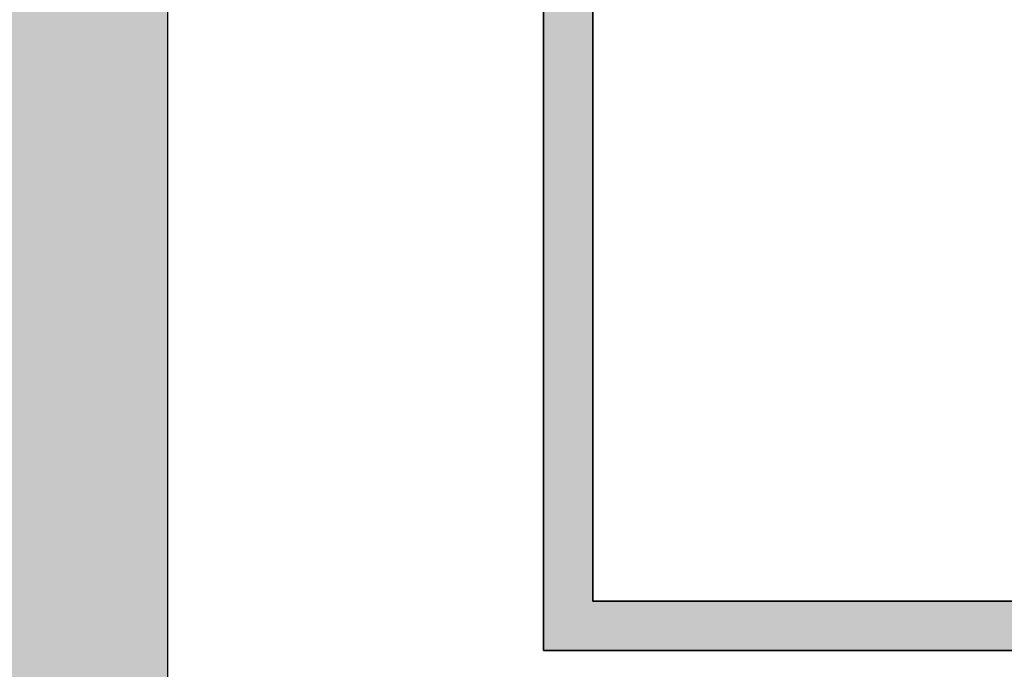
# Model space of a CAD drawing. Units: millimetres. Extents: x -22994 to 29398, y -19990 to 20176.
# Tile 28 of 135: x 99 to 119, y 30 to 43. Entities that reach past the tile are written whole.
import ezdxf
from ezdxf import colors
from ezdxf.entities.mleader import LeaderData, LeaderLine
from ezdxf.math import Vec2, Vec3

# ---------------------------------------------------------------- set-up
doc = ezdxf.new("R2010")
doc.units = ezdxf.units.MM
doc.header["$MEASUREMENT"] = 0
for name, color, linetype, lineweight in [('M-ANNO-TEXT', 7, 'Continuous', 25), ('M-DIMS', 2, 'Continuous', 18), ('M-EQPM', 7, 'Continuous', 25), ('M-EQPM-PATT', 7, 'Continuous', 18), ('M-PIPE', 7, 'Continuous', 35)]:
    doc.layers.add(name, color=color, linetype=linetype, lineweight=lineweight)
doc.styles.get("Standard").update_dxf_attribs({"font": 'arial.ttf'})
doc.dimstyles.get("Standard").update_dxf_attribs({"dimtxt": 0.18, "dimasz": 10000, "dimexe": 0.18, "dimexo": 0.0625, "dimgap": 0.09, "dimtad": 0, "dimtih": 1, "dimtoh": 1, "dimdec": 0, "dimzin": 0, "dimdsep": 46, "dimtxsty": 'Standard', "dimcen": 0.09, "dimadec": 0, "dimazin": 0, "dimtfac": 1, "dimtdec": 0, "dimtofl": 0, "dimtmove": 0, "dimatfit": 3, "dimfxl": 1, "dimtolj": 1, "dimtzin": 0, "dimlwd": 30, "dimarcsym": 0})

# ---------------------------------------------------------------- blocks, each defined once
blk = doc.blocks.new('*D2')
at = {"layer": 'Defpoints', "color": 0, "transparency": 16777216}
for p in [(6.677, 10.271), (290.852, 10.271), (290.852, -5.079)]:
    blk.add_point(p, dxfattribs=at)
at = {"layer": 'M-DIMS', "color": 0, "lineweight": -2, "transparency": 16777216}
for p, q in [((6.677, 10.209), (6.677, -5.259)), ((290.852, 10.209), (290.852, -5.259))]:
    blk.add_line(p, q, dxfattribs=at)
at = {"layer": 'M-DIMS', "color": 0, "lineweight": 30, "transparency": 16777216}
for p, q in [((-9993.323, -5.079), (-19993.323, -5.079)), ((10290.852, -5.079), (20290.852, -5.079))]:
    blk.add_line(p, q, dxfattribs=at)
at = {"layer": 'M-DIMS', "color": 0, "transparency": 16777216}
for points in [[(-9993.323, 1661.588), (-9993.323, -1671.745), (6.677, -5.079)], [(10290.852, 1661.588), (10290.852, -1671.745), (290.852, -5.079)]]:
    blk.add_solid(points, dxfattribs=at)
at = {"layer": 'M-DIMS', "color": 0, "transparency": 16777216, "insert": (148.765, -5.079), "char_height": 0.18, "attachment_point": 5}
blk.add_mtext('\\A1;284.2', dxfattribs=at)
blk = doc.blocks.new('*D3')
at = {"layer": 'Defpoints', "color": 0, "transparency": 16777216}
for p in [(110.265, 204.165), (110.265, 176.366), (95.833, 127.967)]:
    blk.add_point(p, dxfattribs=at)
at = {"layer": 'M-DIMS', "color": 0, "lineweight": -2, "transparency": 16777216}
for p, q in [((95.833, 128.03), (95.833, 204.345)), ((110.265, 176.429), (110.265, 204.345))]:
    blk.add_line(p, q, dxfattribs=at)
at = {"layer": 'M-DIMS', "color": 0, "lineweight": 30, "transparency": 16777216}
for p, q in [((-9904.167, 204.165), (-19904.167, 204.165)), ((10110.265, 204.165), (20110.265, 204.165))]:
    blk.add_line(p, q, dxfattribs=at)
at = {"layer": 'M-DIMS', "color": 0, "transparency": 16777216}
for points in [[(-9904.167, 1870.832), (-9904.167, -1462.501), (95.833, 204.165)], [(10110.265, 1870.832), (10110.265, -1462.501), (110.265, 204.165)]]:
    blk.add_solid(points, dxfattribs=at)
at = {"layer": 'M-DIMS', "color": 0, "transparency": 16777216, "insert": (103.049, 204.165), "char_height": 0.18, "attachment_point": 5}
blk.add_mtext('\\A1;14.432', dxfattribs=at)
blk = doc.blocks.new('*D4')
at = {"layer": 'Defpoints', "color": 0, "transparency": 16777216}
for p in [(116.265, 204.165), (110.265, 176.366), (116.265, 176.366)]:
    blk.add_point(p, dxfattribs=at)
at = {"layer": 'M-DIMS', "color": 0, "lineweight": -2, "transparency": 16777216}
for p, q in [((110.265, 176.429), (110.265, 204.345)), ((116.265, 176.429), (116.265, 204.345))]:
    blk.add_line(p, q, dxfattribs=at)
at = {"layer": 'M-DIMS', "color": 0, "lineweight": 30, "transparency": 16777216}
for p, q in [((-9889.735, 204.165), (-19889.735, 204.165)), ((10116.265, 204.165), (20116.265, 204.165))]:
    blk.add_line(p, q, dxfattribs=at)
at = {"layer": 'M-DIMS', "color": 0, "transparency": 16777216}
for points in [[(-9889.735, 1870.832), (-9889.735, -1462.501), (110.265, 204.165)], [(10116.265, 1870.832), (10116.265, -1462.501), (116.265, 204.165)]]:
    blk.add_solid(points, dxfattribs=at)
at = {"layer": 'M-DIMS', "color": 0, "transparency": 16777216, "insert": (113.265, 204.165), "char_height": 0.18, "attachment_point": 5}
blk.add_mtext('\\A1;6', dxfattribs=at)
blk = doc.blocks.new('*D5')
at = {"layer": 'Defpoints', "color": 0, "transparency": 16777216}
for p in [(181.265, 204.165), (116.265, 176.366), (181.265, 176.366)]:
    blk.add_point(p, dxfattribs=at)
at = {"layer": 'M-DIMS', "color": 0, "lineweight": -2, "transparency": 16777216}
for p, q in [((116.265, 176.429), (116.265, 204.345)), ((181.265, 176.429), (181.265, 204.345))]:
    blk.add_line(p, q, dxfattribs=at)
at = {"layer": 'M-DIMS', "color": 0, "lineweight": 30, "transparency": 16777216}
for p, q in [((-9883.735, 204.165), (-19883.735, 204.165)), ((10181.265, 204.165), (20181.265, 204.165))]:
    blk.add_line(p, q, dxfattribs=at)
at = {"layer": 'M-DIMS', "color": 0, "transparency": 16777216}
for points in [[(-9883.735, 1870.832), (-9883.735, -1462.501), (116.265, 204.165)], [(10181.265, 1870.832), (10181.265, -1462.501), (181.265, 204.165)]]:
    blk.add_solid(points, dxfattribs=at)
at = {"layer": 'M-DIMS', "color": 0, "transparency": 16777216, "insert": (148.765, 204.165), "char_height": 0.18, "attachment_point": 5}
blk.add_mtext('\\A1;65', dxfattribs=at)
blk = doc.blocks.new('*D6')
at = {"layer": 'Defpoints', "color": 0, "transparency": 16777216}
for p in [(187.265, 204.165), (181.265, 176.366), (187.265, 176.366)]:
    blk.add_point(p, dxfattribs=at)
at = {"layer": 'M-DIMS', "color": 0, "lineweight": -2, "transparency": 16777216}
for p, q in [((181.265, 176.429), (181.265, 204.345)), ((187.265, 176.429), (187.265, 204.345))]:
    blk.add_line(p, q, dxfattribs=at)
at = {"layer": 'M-DIMS', "color": 0, "lineweight": 30, "transparency": 16777216}
for p, q in [((-9818.735, 204.165), (-19818.735, 204.165)), ((10187.265, 204.165), (20187.265, 204.165))]:
    blk.add_line(p, q, dxfattribs=at)
at = {"layer": 'M-DIMS', "color": 0, "transparency": 16777216}
for points in [[(-9818.735, 1870.832), (-9818.735, -1462.501), (181.265, 204.165)], [(10187.265, 1870.832), (10187.265, -1462.501), (187.265, 204.165)]]:
    blk.add_solid(points, dxfattribs=at)
at = {"layer": 'M-DIMS', "color": 0, "transparency": 16777216, "insert": (184.265, 204.165), "char_height": 0.18, "attachment_point": 5}
blk.add_mtext('\\A1;6', dxfattribs=at)
blk = doc.blocks.new('*D7')
at = {"layer": 'Defpoints', "color": 0, "transparency": 16777216}
for p in [(201.697, 204.165), (187.265, 176.366), (201.697, 127.967)]:
    blk.add_point(p, dxfattribs=at)
at = {"layer": 'M-DIMS', "color": 0, "lineweight": -2, "transparency": 16777216}
for p, q in [((187.265, 176.429), (187.265, 204.345)), ((201.697, 128.03), (201.697, 204.345))]:
    blk.add_line(p, q, dxfattribs=at)
at = {"layer": 'M-DIMS', "color": 0, "lineweight": 30, "transparency": 16777216}
for p, q in [((-9812.735, 204.165), (-19812.735, 204.165)), ((10201.697, 204.165), (20201.697, 204.165))]:
    blk.add_line(p, q, dxfattribs=at)
at = {"layer": 'M-DIMS', "color": 0, "transparency": 16777216}
for points in [[(-9812.735, 1870.832), (-9812.735, -1462.501), (187.265, 204.165)], [(10201.697, 1870.832), (10201.697, -1462.501), (201.697, 204.165)]]:
    blk.add_solid(points, dxfattribs=at)
at = {"layer": 'M-DIMS', "color": 0, "transparency": 16777216, "insert": (194.481, 204.165), "char_height": 0.18, "attachment_point": 5}
blk.add_mtext('\\A1;14.432', dxfattribs=at)
blk = doc.blocks.new('*D8')
at = {"layer": 'Defpoints', "color": 0, "transparency": 16777216}
for p in [(227.648, 204.165), (227.648, 146.73), (201.697, 127.967)]:
    blk.add_point(p, dxfattribs=at)
at = {"layer": 'M-DIMS', "color": 0, "lineweight": -2, "transparency": 16777216}
for p, q in [((201.697, 128.03), (201.697, 204.345)), ((227.648, 146.792), (227.648, 204.345))]:
    blk.add_line(p, q, dxfattribs=at)
at = {"layer": 'M-DIMS', "color": 0, "lineweight": 30, "transparency": 16777216}
for p, q in [((-9798.303, 204.165), (-19798.303, 204.165)), ((10227.648, 204.165), (20227.648, 204.165))]:
    blk.add_line(p, q, dxfattribs=at)
at = {"layer": 'M-DIMS', "color": 0, "transparency": 16777216}
for points in [[(-9798.303, 1870.832), (-9798.303, -1462.501), (201.697, 204.165)], [(10227.648, 1870.832), (10227.648, -1462.501), (227.648, 204.165)]]:
    blk.add_solid(points, dxfattribs=at)
at = {"layer": 'M-DIMS', "color": 0, "transparency": 16777216, "insert": (214.673, 204.165), "char_height": 0.18, "attachment_point": 5}
blk.add_mtext('\\A1;25.95', dxfattribs=at)
blk = doc.blocks.new('*D9')
at = {"layer": 'Defpoints', "color": 0, "transparency": 16777216}
for p in [(187.265, 176.366), (306.202, 176.366), (290.852, 10.271)]:
    blk.add_point(p, dxfattribs=at)
at = {"layer": 'M-DIMS', "color": 0, "lineweight": 30, "transparency": 16777216}
for p, q in [((306.202, 10176.366), (306.202, 20176.366)), ((306.202, -9989.729), (306.202, -19989.729))]:
    blk.add_line(p, q, dxfattribs=at)
at = {"layer": 'M-DIMS', "color": 0, "lineweight": -2, "transparency": 16777216}
for p, q in [((187.327, 176.366), (306.382, 176.366)), ((290.915, 10.271), (306.382, 10.271))]:
    blk.add_line(p, q, dxfattribs=at)
at = {"layer": 'M-DIMS', "color": 0, "transparency": 16777216}
for points in [[(-1360.465, 10176.366), (1972.869, 10176.366), (306.202, 176.366)], [(-1360.465, -9989.729), (1972.869, -9989.729), (306.202, 10.271)]]:
    blk.add_solid(points, dxfattribs=at)
at = {"layer": 'M-DIMS', "color": 0, "transparency": 16777216, "insert": (306.202, 93.319), "char_height": 0.18, "attachment_point": 5}
blk.add_mtext('\\A1;166.1', dxfattribs=at)
blk = doc.blocks.new('*D10')
at = {"layer": 'Defpoints', "color": 0, "transparency": 16777216}
for p in [(125.65, 136.071), (133.346, 136.071), (133.346, -5.079)]:
    blk.add_point(p, dxfattribs=at)
at = {"layer": 'M-DIMS', "color": 0, "lineweight": -2, "transparency": 16777216}
for p, q in [((125.65, 136.009), (125.65, -5.259)), ((133.346, 136.009), (133.346, -5.259))]:
    blk.add_line(p, q, dxfattribs=at)
at = {"layer": 'M-DIMS', "color": 0, "lineweight": 30, "transparency": 16777216}
for p, q in [((-9874.35, -5.079), (-19874.35, -5.079)), ((10133.346, -5.079), (20133.346, -5.079))]:
    blk.add_line(p, q, dxfattribs=at)
at = {"layer": 'M-DIMS', "color": 0, "transparency": 16777216}
for points in [[(-9874.35, 1661.588), (-9874.35, -1671.745), (125.65, -5.079)], [(10133.346, 1661.588), (10133.346, -1671.745), (133.346, -5.079)]]:
    blk.add_solid(points, dxfattribs=at)
at = {"layer": 'M-DIMS', "color": 0, "transparency": 16777216, "insert": (129.498, -5.079), "char_height": 0.18, "attachment_point": 5}
blk.add_mtext('\\A1;7.696', dxfattribs=at)
blk = doc.blocks.new('*D11')
at = {"layer": 'Defpoints', "color": 0, "transparency": 16777216}
for p in [(133.346, 136.071), (135.65, 136.071), (135.65, -5.079)]:
    blk.add_point(p, dxfattribs=at)
at = {"layer": 'M-DIMS', "color": 0, "lineweight": -2, "transparency": 16777216}
for p, q in [((133.346, 136.009), (133.346, -5.259)), ((135.65, 136.009), (135.65, -5.259))]:
    blk.add_line(p, q, dxfattribs=at)
at = {"layer": 'M-DIMS', "color": 0, "lineweight": 30, "transparency": 16777216}
for p, q in [((-9866.654, -5.079), (-19866.654, -5.079)), ((10135.65, -5.079), (20135.65, -5.079))]:
    blk.add_line(p, q, dxfattribs=at)
at = {"layer": 'M-DIMS', "color": 0, "transparency": 16777216}
for points in [[(-9866.654, 1661.588), (-9866.654, -1671.745), (133.346, -5.079)], [(10135.65, 1661.588), (10135.65, -1671.745), (135.65, -5.079)]]:
    blk.add_solid(points, dxfattribs=at)
at = {"layer": 'M-DIMS', "color": 0, "transparency": 16777216, "insert": (134.498, -5.079), "char_height": 0.18, "attachment_point": 5}
blk.add_mtext('\\A1;2.304', dxfattribs=at)
blk = doc.blocks.new('*D12')
at = {"layer": 'Defpoints', "color": 0, "transparency": 16777216}
for p in [(135.65, 136.071), (145.65, 136.071), (145.65, -5.079)]:
    blk.add_point(p, dxfattribs=at)
at = {"layer": 'M-DIMS', "color": 0, "lineweight": -2, "transparency": 16777216}
for p, q in [((135.65, 136.009), (135.65, -5.259)), ((145.65, 136.009), (145.65, -5.259))]:
    blk.add_line(p, q, dxfattribs=at)
at = {"layer": 'M-DIMS', "color": 0, "lineweight": 30, "transparency": 16777216}
for p, q in [((-9864.35, -5.079), (-19864.35, -5.079)), ((10145.65, -5.079), (20145.65, -5.079))]:
    blk.add_line(p, q, dxfattribs=at)
at = {"layer": 'M-DIMS', "color": 0, "transparency": 16777216}
for points in [[(-9864.35, 1661.588), (-9864.35, -1671.745), (135.65, -5.079)], [(10145.65, 1661.588), (10145.65, -1671.745), (145.65, -5.079)]]:
    blk.add_solid(points, dxfattribs=at)
at = {"layer": 'M-DIMS', "color": 0, "transparency": 16777216, "insert": (140.65, -5.079), "char_height": 0.18, "attachment_point": 5}
blk.add_mtext('\\A1;10', dxfattribs=at)
blk = doc.blocks.new('*D13')
at = {"layer": 'Defpoints', "color": 0, "transparency": 16777216}
for p in [(145.65, 136.071), (155.65, 136.071), (155.65, -5.079)]:
    blk.add_point(p, dxfattribs=at)
at = {"layer": 'M-DIMS', "color": 0, "lineweight": -2, "transparency": 16777216}
for p, q in [((145.65, 136.009), (145.65, -5.259)), ((155.65, 136.009), (155.65, -5.259))]:
    blk.add_line(p, q, dxfattribs=at)
at = {"layer": 'M-DIMS', "color": 0, "lineweight": 30, "transparency": 16777216}
for p, q in [((-9854.35, -5.079), (-19854.35, -5.079)), ((10155.65, -5.079), (20155.65, -5.079))]:
    blk.add_line(p, q, dxfattribs=at)
at = {"layer": 'M-DIMS', "color": 0, "transparency": 16777216}
for points in [[(-9854.35, 1661.588), (-9854.35, -1671.745), (145.65, -5.079)], [(10155.65, 1661.588), (10155.65, -1671.745), (155.65, -5.079)]]:
    blk.add_solid(points, dxfattribs=at)
at = {"layer": 'M-DIMS', "color": 0, "transparency": 16777216, "insert": (150.65, -5.079), "char_height": 0.18, "attachment_point": 5}
blk.add_mtext('\\A1;10', dxfattribs=at)
blk = doc.blocks.new('*D14')
at = {"layer": 'Defpoints', "color": 0, "transparency": 16777216}
for p in [(155.65, 136.071), (165.65, 136.071), (165.65, -5.079)]:
    blk.add_point(p, dxfattribs=at)
at = {"layer": 'M-DIMS', "color": 0, "lineweight": -2, "transparency": 16777216}
for p, q in [((155.65, 136.009), (155.65, -5.259)), ((165.65, 136.009), (165.65, -5.259))]:
    blk.add_line(p, q, dxfattribs=at)
at = {"layer": 'M-DIMS', "color": 0, "lineweight": 30, "transparency": 16777216}
for p, q in [((-9844.35, -5.079), (-19844.35, -5.079)), ((10165.65, -5.079), (20165.65, -5.079))]:
    blk.add_line(p, q, dxfattribs=at)
at = {"layer": 'M-DIMS', "color": 0, "transparency": 16777216}
for points in [[(-9844.35, 1661.588), (-9844.35, -1671.745), (155.65, -5.079)], [(10165.65, 1661.588), (10165.65, -1671.745), (165.65, -5.079)]]:
    blk.add_solid(points, dxfattribs=at)
at = {"layer": 'M-DIMS', "color": 0, "transparency": 16777216, "insert": (160.65, -5.079), "char_height": 0.18, "attachment_point": 5}
blk.add_mtext('\\A1;10', dxfattribs=at)
blk = doc.blocks.new('*D15')
at = {"layer": 'Defpoints', "color": 0, "transparency": 16777216}
for p in [(173.346, 154.788), (173.346, 136.071), (306.202, 136.071)]:
    blk.add_point(p, dxfattribs=at)
at = {"layer": 'M-DIMS', "color": 0, "lineweight": 30, "transparency": 16777216}
for p, q in [((306.202, 10154.788), (306.202, 20154.788)), ((306.202, -9863.929), (306.202, -19863.929))]:
    blk.add_line(p, q, dxfattribs=at)
at = {"layer": 'M-DIMS', "color": 0, "lineweight": -2, "transparency": 16777216}
for p, q in [((173.408, 154.788), (306.382, 154.788)), ((173.408, 136.071), (306.382, 136.071))]:
    blk.add_line(p, q, dxfattribs=at)
at = {"layer": 'M-DIMS', "color": 0, "transparency": 16777216}
for points in [[(-1360.465, 10154.788), (1972.869, 10154.788), (306.202, 154.788)], [(-1360.465, -9863.929), (1972.869, -9863.929), (306.202, 136.071)]]:
    blk.add_solid(points, dxfattribs=at)
at = {"layer": 'M-DIMS', "color": 0, "transparency": 16777216, "insert": (306.202, 145.43), "char_height": 0.18, "attachment_point": 5}
blk.add_mtext('\\A1;18.717', dxfattribs=at)
blk = doc.blocks.new('*D16')
at = {"layer": 'Defpoints', "color": 0, "transparency": 16777216}
for p in [(120.17, 204.165), (110.466, 48.035), (120.17, 48.035)]:
    blk.add_point(p, dxfattribs=at)
at = {"layer": 'M-DIMS', "color": 0, "lineweight": -2, "transparency": 16777216}
for p, q in [((110.466, 48.097), (110.466, 204.345)), ((120.17, 48.097), (120.17, 204.345))]:
    blk.add_line(p, q, dxfattribs=at)
at = {"layer": 'M-DIMS', "color": 0, "lineweight": 30, "transparency": 16777216}
for p, q in [((-9889.534, 204.165), (-19889.534, 204.165)), ((10120.17, 204.165), (20120.17, 204.165))]:
    blk.add_line(p, q, dxfattribs=at)
at = {"layer": 'M-DIMS', "color": 0, "transparency": 16777216}
for points in [[(-9889.534, 1870.832), (-9889.534, -1462.501), (110.466, 204.165)], [(10120.17, 1870.832), (10120.17, -1462.501), (120.17, 204.165)]]:
    blk.add_solid(points, dxfattribs=at)
at = {"layer": 'M-DIMS', "color": 0, "transparency": 16777216, "insert": (115.318, 204.165), "char_height": 0.18, "attachment_point": 5}
blk.add_mtext('\\A1;9.704', dxfattribs=at)
blk = doc.blocks.new('*D17')
at = {"layer": 'Defpoints', "color": 0, "transparency": 16777216}
for p in [(126.17, 204.165), (120.17, 48.035), (126.17, 48.035)]:
    blk.add_point(p, dxfattribs=at)
at = {"layer": 'M-DIMS', "color": 0, "lineweight": -2, "transparency": 16777216}
for p, q in [((120.17, 48.097), (120.17, 204.345)), ((126.17, 48.097), (126.17, 204.345))]:
    blk.add_line(p, q, dxfattribs=at)
at = {"layer": 'M-DIMS', "color": 0, "lineweight": 30, "transparency": 16777216}
for p, q in [((-9879.83, 204.165), (-19879.83, 204.165)), ((10126.17, 204.165), (20126.17, 204.165))]:
    blk.add_line(p, q, dxfattribs=at)
at = {"layer": 'M-DIMS', "color": 0, "transparency": 16777216}
for points in [[(-9879.83, 1870.832), (-9879.83, -1462.501), (120.17, 204.165)], [(10126.17, 1870.832), (10126.17, -1462.501), (126.17, 204.165)]]:
    blk.add_solid(points, dxfattribs=at)
at = {"layer": 'M-DIMS', "color": 0, "transparency": 16777216, "insert": (123.17, 204.165), "char_height": 0.18, "attachment_point": 5}
blk.add_mtext('\\A1;6', dxfattribs=at)
blk = doc.blocks.new('*D18')
at = {"layer": 'Defpoints', "color": 0, "transparency": 16777216}
for p in [(132.17, 204.165), (126.17, 48.035), (132.17, 48.035)]:
    blk.add_point(p, dxfattribs=at)
at = {"layer": 'M-DIMS', "color": 0, "lineweight": -2, "transparency": 16777216}
for p, q in [((126.17, 48.097), (126.17, 204.345)), ((132.17, 48.097), (132.17, 204.345))]:
    blk.add_line(p, q, dxfattribs=at)
at = {"layer": 'M-DIMS', "color": 0, "lineweight": 30, "transparency": 16777216}
for p, q in [((-9873.83, 204.165), (-19873.83, 204.165)), ((10132.17, 204.165), (20132.17, 204.165))]:
    blk.add_line(p, q, dxfattribs=at)
at = {"layer": 'M-DIMS', "color": 0, "transparency": 16777216}
for points in [[(-9873.83, 1870.832), (-9873.83, -1462.501), (126.17, 204.165)], [(10132.17, 1870.832), (10132.17, -1462.501), (132.17, 204.165)]]:
    blk.add_solid(points, dxfattribs=at)
at = {"layer": 'M-DIMS', "color": 0, "transparency": 16777216, "insert": (129.17, 204.165), "char_height": 0.18, "attachment_point": 5}
blk.add_mtext('\\A1;6', dxfattribs=at)
blk = doc.blocks.new('*D19')
at = {"layer": 'Defpoints', "color": 0, "transparency": 16777216}
for p in [(138.17, 204.165), (132.17, 48.035), (138.17, 48.035)]:
    blk.add_point(p, dxfattribs=at)
at = {"layer": 'M-DIMS', "color": 0, "lineweight": -2, "transparency": 16777216}
for p, q in [((132.17, 48.097), (132.17, 204.345)), ((138.17, 48.097), (138.17, 204.345))]:
    blk.add_line(p, q, dxfattribs=at)
at = {"layer": 'M-DIMS', "color": 0, "lineweight": 30, "transparency": 16777216}
for p, q in [((-9867.83, 204.165), (-19867.83, 204.165)), ((10138.17, 204.165), (20138.17, 204.165))]:
    blk.add_line(p, q, dxfattribs=at)
at = {"layer": 'M-DIMS', "color": 0, "transparency": 16777216}
for points in [[(-9867.83, 1870.832), (-9867.83, -1462.501), (132.17, 204.165)], [(10138.17, 1870.832), (10138.17, -1462.501), (138.17, 204.165)]]:
    blk.add_solid(points, dxfattribs=at)
at = {"layer": 'M-DIMS', "color": 0, "transparency": 16777216, "insert": (135.17, 204.165), "char_height": 0.18, "attachment_point": 5}
blk.add_mtext('\\A1;6', dxfattribs=at)
blk = doc.blocks.new('*D20')
at = {"layer": 'Defpoints', "color": 0, "transparency": 16777216}
for p in [(144.17, 204.165), (138.17, 48.035), (144.17, 48.035)]:
    blk.add_point(p, dxfattribs=at)
at = {"layer": 'M-DIMS', "color": 0, "lineweight": -2, "transparency": 16777216}
for p, q in [((138.17, 48.097), (138.17, 204.345)), ((144.17, 48.097), (144.17, 204.345))]:
    blk.add_line(p, q, dxfattribs=at)
at = {"layer": 'M-DIMS', "color": 0, "lineweight": 30, "transparency": 16777216}
for p, q in [((-9861.83, 204.165), (-19861.83, 204.165)), ((10144.17, 204.165), (20144.17, 204.165))]:
    blk.add_line(p, q, dxfattribs=at)
at = {"layer": 'M-DIMS', "color": 0, "transparency": 16777216}
for points in [[(-9861.83, 1870.832), (-9861.83, -1462.501), (138.17, 204.165)], [(10144.17, 1870.832), (10144.17, -1462.501), (144.17, 204.165)]]:
    blk.add_solid(points, dxfattribs=at)
at = {"layer": 'M-DIMS', "color": 0, "transparency": 16777216, "insert": (141.17, 204.165), "char_height": 0.18, "attachment_point": 5}
blk.add_mtext('\\A1;6', dxfattribs=at)
blk = doc.blocks.new('*D21')
at = {"layer": 'Defpoints', "color": 0, "transparency": 16777216}
for p in [(149.116, 204.165), (144.17, 48.035), (149.116, 48.035)]:
    blk.add_point(p, dxfattribs=at)
at = {"layer": 'M-DIMS', "color": 0, "lineweight": -2, "transparency": 16777216}
for p, q in [((144.17, 48.097), (144.17, 204.345)), ((149.116, 48.097), (149.116, 204.345))]:
    blk.add_line(p, q, dxfattribs=at)
at = {"layer": 'M-DIMS', "color": 0, "lineweight": 30, "transparency": 16777216}
for p, q in [((-9855.83, 204.165), (-19855.83, 204.165)), ((10149.116, 204.165), (20149.116, 204.165))]:
    blk.add_line(p, q, dxfattribs=at)
at = {"layer": 'M-DIMS', "color": 0, "transparency": 16777216}
for points in [[(-9855.83, 1870.832), (-9855.83, -1462.501), (144.17, 204.165)], [(10149.116, 1870.832), (10149.116, -1462.501), (149.116, 204.165)]]:
    blk.add_solid(points, dxfattribs=at)
at = {"layer": 'M-DIMS', "color": 0, "transparency": 16777216, "insert": (146.643, 204.165), "char_height": 0.18, "attachment_point": 5}
blk.add_mtext('\\A1;4.945', dxfattribs=at)
blk = doc.blocks.new('*D22')
at = {"layer": 'Defpoints', "color": 0, "transparency": 16777216}
for p in [(149.116, 30.99), (155.116, 30.99), (155.116, -5.079)]:
    blk.add_point(p, dxfattribs=at)
at = {"layer": 'M-DIMS', "color": 0, "lineweight": -2, "transparency": 16777216}
for p, q in [((149.116, 30.927), (149.116, -5.259)), ((155.116, 30.927), (155.116, -5.259))]:
    blk.add_line(p, q, dxfattribs=at)
at = {"layer": 'M-DIMS', "color": 0, "lineweight": 30, "transparency": 16777216}
for p, q in [((-9850.884, -5.079), (-19850.884, -5.079)), ((10155.116, -5.079), (20155.116, -5.079))]:
    blk.add_line(p, q, dxfattribs=at)
at = {"layer": 'M-DIMS', "color": 0, "transparency": 16777216}
for points in [[(-9850.884, 1661.588), (-9850.884, -1671.745), (149.116, -5.079)], [(10155.116, 1661.588), (10155.116, -1671.745), (155.116, -5.079)]]:
    blk.add_solid(points, dxfattribs=at)
at = {"layer": 'M-DIMS', "color": 0, "transparency": 16777216, "insert": (152.116, -5.079), "char_height": 0.18, "attachment_point": 5}
blk.add_mtext('\\A1;6', dxfattribs=at)
blk = doc.blocks.new('*D23')
at = {"layer": 'Defpoints', "color": 0, "transparency": 16777216}
for p in [(155.116, 30.99), (161.116, 30.99), (161.116, -5.079)]:
    blk.add_point(p, dxfattribs=at)
at = {"layer": 'M-DIMS', "color": 0, "lineweight": -2, "transparency": 16777216}
for p, q in [((155.116, 30.927), (155.116, -5.259)), ((161.116, 30.927), (161.116, -5.259))]:
    blk.add_line(p, q, dxfattribs=at)
at = {"layer": 'M-DIMS', "color": 0, "lineweight": 30, "transparency": 16777216}
for p, q in [((-9844.884, -5.079), (-19844.884, -5.079)), ((10161.116, -5.079), (20161.116, -5.079))]:
    blk.add_line(p, q, dxfattribs=at)
at = {"layer": 'M-DIMS', "color": 0, "transparency": 16777216}
for points in [[(-9844.884, 1661.588), (-9844.884, -1671.745), (155.116, -5.079)], [(10161.116, 1661.588), (10161.116, -1671.745), (161.116, -5.079)]]:
    blk.add_solid(points, dxfattribs=at)
at = {"layer": 'M-DIMS', "color": 0, "transparency": 16777216, "insert": (158.116, -5.079), "char_height": 0.18, "attachment_point": 5}
blk.add_mtext('\\A1;6', dxfattribs=at)
blk = doc.blocks.new('*D24')
at = {"layer": 'Defpoints', "color": 0, "transparency": 16777216}
for p in [(161.116, 30.99), (166.439, 30.99), (166.439, -5.079)]:
    blk.add_point(p, dxfattribs=at)
at = {"layer": 'M-DIMS', "color": 0, "lineweight": -2, "transparency": 16777216}
for p, q in [((161.116, 30.927), (161.116, -5.259)), ((166.439, 30.927), (166.439, -5.259))]:
    blk.add_line(p, q, dxfattribs=at)
at = {"layer": 'M-DIMS', "color": 0, "lineweight": 30, "transparency": 16777216}
for p, q in [((-9838.884, -5.079), (-19838.884, -5.079)), ((10166.439, -5.079), (20166.439, -5.079))]:
    blk.add_line(p, q, dxfattribs=at)
at = {"layer": 'M-DIMS', "color": 0, "transparency": 16777216}
for points in [[(-9838.884, 1661.588), (-9838.884, -1671.745), (161.116, -5.079)], [(10166.439, 1661.588), (10166.439, -1671.745), (166.439, -5.079)]]:
    blk.add_solid(points, dxfattribs=at)
at = {"layer": 'M-DIMS', "color": 0, "transparency": 16777216, "insert": (163.777, -5.079), "char_height": 0.18, "attachment_point": 5}
blk.add_mtext('\\A1;5.323', dxfattribs=at)
blk = doc.blocks.new('*D25')
at = {"layer": 'Defpoints', "color": 0, "transparency": 16777216}
for p in [(166.439, 30.99), (172.439, 30.99), (172.439, -5.079)]:
    blk.add_point(p, dxfattribs=at)
at = {"layer": 'M-DIMS', "color": 0, "lineweight": -2, "transparency": 16777216}
for p, q in [((166.439, 30.927), (166.439, -5.259)), ((172.439, 30.927), (172.439, -5.259))]:
    blk.add_line(p, q, dxfattribs=at)
at = {"layer": 'M-DIMS', "color": 0, "lineweight": 30, "transparency": 16777216}
for p, q in [((-9833.561, -5.079), (-19833.561, -5.079)), ((10172.439, -5.079), (20172.439, -5.079))]:
    blk.add_line(p, q, dxfattribs=at)
at = {"layer": 'M-DIMS', "color": 0, "transparency": 16777216}
for points in [[(-9833.561, 1661.588), (-9833.561, -1671.745), (166.439, -5.079)], [(10172.439, 1661.588), (10172.439, -1671.745), (172.439, -5.079)]]:
    blk.add_solid(points, dxfattribs=at)
at = {"layer": 'M-DIMS', "color": 0, "transparency": 16777216, "insert": (169.439, -5.079), "char_height": 0.18, "attachment_point": 5}
blk.add_mtext('\\A1;6', dxfattribs=at)
blk = doc.blocks.new('*D26')
at = {"layer": 'Defpoints', "color": 0, "transparency": 16777216}
for p in [(172.439, 30.99), (178.439, 30.99), (178.439, -5.079)]:
    blk.add_point(p, dxfattribs=at)
at = {"layer": 'M-DIMS', "color": 0, "lineweight": -2, "transparency": 16777216}
for p, q in [((172.439, 30.927), (172.439, -5.259)), ((178.439, 30.927), (178.439, -5.259))]:
    blk.add_line(p, q, dxfattribs=at)
at = {"layer": 'M-DIMS', "color": 0, "lineweight": 30, "transparency": 16777216}
for p, q in [((-9827.561, -5.079), (-19827.561, -5.079)), ((10178.439, -5.079), (20178.439, -5.079))]:
    blk.add_line(p, q, dxfattribs=at)
at = {"layer": 'M-DIMS', "color": 0, "transparency": 16777216}
for points in [[(-9827.561, 1661.588), (-9827.561, -1671.745), (172.439, -5.079)], [(10178.439, 1661.588), (10178.439, -1671.745), (178.439, -5.079)]]:
    blk.add_solid(points, dxfattribs=at)
at = {"layer": 'M-DIMS', "color": 0, "transparency": 16777216, "insert": (175.439, -5.079), "char_height": 0.18, "attachment_point": 5}
blk.add_mtext('\\A1;6', dxfattribs=at)
blk = doc.blocks.new('*D27')
at = {"layer": 'Defpoints', "color": 0, "transparency": 16777216}
for p in [(178.439, 30.99), (188.117, 30.99), (188.117, -5.079)]:
    blk.add_point(p, dxfattribs=at)
at = {"layer": 'M-DIMS', "color": 0, "lineweight": -2, "transparency": 16777216}
for p, q in [((178.439, 30.927), (178.439, -5.259)), ((188.117, 30.927), (188.117, -5.259))]:
    blk.add_line(p, q, dxfattribs=at)
at = {"layer": 'M-DIMS', "color": 0, "lineweight": 30, "transparency": 16777216}
for p, q in [((-9821.561, -5.079), (-19821.561, -5.079)), ((10188.117, -5.079), (20188.117, -5.079))]:
    blk.add_line(p, q, dxfattribs=at)
at = {"layer": 'M-DIMS', "color": 0, "transparency": 16777216}
for points in [[(-9821.561, 1661.588), (-9821.561, -1671.745), (178.439, -5.079)], [(10188.117, 1661.588), (10188.117, -1671.745), (188.117, -5.079)]]:
    blk.add_solid(points, dxfattribs=at)
at = {"layer": 'M-DIMS', "color": 0, "transparency": 16777216, "insert": (183.278, -5.079), "char_height": 0.18, "attachment_point": 5}
blk.add_mtext('\\A1;9.679', dxfattribs=at)
blk = doc.blocks.new('*D28')
at = {"layer": 'Defpoints', "color": 0, "transparency": 16777216}
for p in [(188.117, 48.035), (306.202, 48.035), (188.117, 30.99)]:
    blk.add_point(p, dxfattribs=at)
at = {"layer": 'M-DIMS', "color": 0, "lineweight": 30, "transparency": 16777216}
for p, q in [((306.202, 10048.035), (306.202, 20048.035)), ((306.202, -9969.01), (306.202, -19969.01))]:
    blk.add_line(p, q, dxfattribs=at)
at = {"layer": 'M-DIMS', "color": 0, "lineweight": -2, "transparency": 16777216}
for p, q in [((188.18, 48.035), (306.382, 48.035)), ((188.18, 30.99), (306.382, 30.99))]:
    blk.add_line(p, q, dxfattribs=at)
at = {"layer": 'M-DIMS', "color": 0, "transparency": 16777216}
for points in [[(-1360.465, 10048.035), (1972.869, 10048.035), (306.202, 48.035)], [(-1360.465, -9969.01), (1972.869, -9969.01), (306.202, 30.99)]]:
    blk.add_solid(points, dxfattribs=at)
at = {"layer": 'M-DIMS', "color": 0, "transparency": 16777216, "insert": (306.202, 39.512), "char_height": 0.18, "attachment_point": 5}
blk.add_mtext('\\A1;17.045', dxfattribs=at)
blk = doc.blocks.new('*D29')
at = {"layer": 'Defpoints', "color": 0, "transparency": 16777216}
for p in [(36.801, 80.045), (64.03, 80.045)]:
    blk.add_point(p, dxfattribs=at)
at = {"layer": 'M-DIMS', "color": 0, "lineweight": -2, "transparency": 16777216}
for p, q in [((50.415, 79.955), (50.415, 80.135)), ((50.325, 80.045), (50.505, 80.045))]:
    blk.add_line(p, q, dxfattribs=at)
at = {"layer": 'M-DIMS', "color": 0, "lineweight": 30, "transparency": 16777216}
blk.add_line((20064.03, 80.03), (10064.03, 80.038), dxfattribs=at)
at = {"layer": 'M-DIMS', "color": 0, "transparency": 16777216}
blk.add_solid([(10064.031, 1746.704), (10064.028, -1586.629), (64.03, 80.045)], dxfattribs=at)
at = {"layer": 'M-DIMS', "color": 0, "transparency": 16777216, "insert": (20064.521, 80.03), "char_height": 0.18, "attachment_point": 5}
blk.add_mtext('\\A1;∅27.23', dxfattribs=at)
blk = doc.blocks.new('*D36')
at = {"layer": 'Defpoints', "color": 0, "transparency": 16777216}
for p in [(46.39, 31.303), (46.387, 26.593)]:
    blk.add_point(p, dxfattribs=at)
at = {"layer": 'M-DIMS', "color": 0, "lineweight": 30, "transparency": 16777216}
for p, q in [((57.15, 20031.301), (51.77, 10031.302)), ((10057.15, 20031.301), (57.15, 20031.301))]:
    blk.add_line(p, q, dxfattribs=at)
at = {"layer": 'M-DIMS', "color": 0, "lineweight": -2, "transparency": 16777216}
for p, q in [((46.389, 28.858), (46.389, 29.038)), ((46.299, 28.948), (46.479, 28.948))]:
    blk.add_line(p, q, dxfattribs=at)
at = {"layer": 'M-DIMS', "color": 0, "transparency": 16777216}
blk.add_solid([(-1614.896, 10032.199), (1718.436, 10030.405), (46.39, 31.303)], dxfattribs=at)
at = {"layer": 'M-DIMS', "color": 0, "transparency": 16777216, "insert": (10057.554, 20031.301), "char_height": 0.18, "attachment_point": 5}
blk.add_mtext('\\A1;∅4.71', dxfattribs=at)
blk = doc.blocks.new('*D37')
at = {"layer": 'Defpoints', "color": 0, "transparency": 16777216}
for p in [(54.834, 118.615), (59.494, 118.614)]:
    blk.add_point(p, dxfattribs=at)
at = {"layer": 'M-DIMS', "color": 0, "lineweight": -2, "transparency": 16777216}
for p, q in [((57.164, 118.524), (57.164, 118.704)), ((57.074, 118.614), (57.254, 118.614))]:
    blk.add_line(p, q, dxfattribs=at)
at = {"layer": 'M-DIMS', "color": 0, "lineweight": 30, "transparency": 16777216}
blk.add_line((20059.493, 116.253), (10059.494, 117.434), dxfattribs=at)
at = {"layer": 'M-DIMS', "color": 0, "transparency": 16777216}
blk.add_solid([(10059.69, 1784.1), (10059.297, -1549.233), (59.494, 118.614)], dxfattribs=at)
at = {"layer": 'M-DIMS', "color": 0, "transparency": 16777216, "insert": (20059.985, 116.253), "char_height": 0.18, "attachment_point": 5}
blk.add_mtext('\\A1;∅4.659', dxfattribs=at)

msp = doc.modelspace()

# ---------------------------------------------------------------- hatches: boundary and pattern name
at = {"layer": 'M-EQPM-PATT'}
h = msp.add_hatch(color=256, dxfattribs=at)
h.set_gradient(color1=(205, 32, 39), color2=(205, 32, 39), tint=1)
h.paths.add_polyline_path([(116.2647, 150.3662), (116.2647, 170.3662), (116.2647, 176.3662), (110.2647, 176.3662), (110.2647, 152.0276), (95.8327, 127.967), (95.8327, 16.6063), (201.6967, 16.6063), (201.6967, 127.967), (187.2647, 152.0276), (187.2647, 176.3662), (181.2647, 176.3662), (181.2647, 170.3662), (181.2647, 150.3662), (195.6967, 126.3055), (195.6967, 22.6063), (101.8327, 22.6063), (101.8327, 126.3055)])
h.paths.add_polyline_path([(185.2208, 88.6347), (101.8327, 88.6347), (101.8327, 87.6347), (182.8066, 87.6347), (178.7313, 83.5594), (195.6967, 83.5594), (195.6967, 84.5594), (181.1455, 84.5594)], flags=17)
h.paths.add_polyline_path([(95.8327, 88.6347), (60.9779, 88.6347, -0.0228552), (61.7178, 87.6347), (95.8327, 87.6347)])
h.paths.add_polyline_path([(215.6212, 86.5189), (215.6212, 80.5999), (220.5095, 83.5594)])
h.paths.add_polyline_path([(215.6212, 84.5594), (201.6967, 84.5594), (201.6967, 83.5594), (215.6212, 83.5594)])
h.paths.add_polyline_path([(225.3978, 86.5189), (220.5095, 83.5594), (225.3978, 80.5999)])
h.paths.add_polyline_path([(231.6256, 84.5594), (225.3978, 84.5594), (225.3978, 83.5594), (231.6256, 83.5594)])
h = msp.add_hatch(color=256, dxfattribs=at)
h.set_gradient(color1=(19, 155, 72), color2=(88, 186, 72), tint=1, name='CYLINDER')
h.paths.add_polyline_path([(109.4658, 29.9895), (189.1175, 29.9895), (189.1175, 77.6953), (128.1172, 77.6953, 0.4142136), (126.1172, 75.6953), (126.1172, 73.6953, 0.4142136), (128.1172, 71.6953), (178.5136, 71.6953, -0.4142136), (179.5136, 70.6953), (179.5136, 68.6953, -0.4142136), (178.5136, 67.6953), (128.1172, 67.6953, 0.4142136), (126.1172, 65.6953), (126.1172, 63.6953, 0.4142136), (128.1172, 61.6953), (178.5136, 61.6953, -0.4142136), (179.5136, 60.6953), (179.5136, 58.6953, -0.4142136), (178.5136, 57.6953), (109.7466, 57.6953, -0.4142136), (108.7466, 58.6953), (108.7466, 75.5922, 0.4142136), (106.7466, 77.5922), (101.8327, 77.5922), (101.8327, 76.5922), (106.7466, 76.5922, -0.4142136), (107.7466, 75.5922), (107.7466, 58.6953, 0.4142136), (109.7466, 56.6953), (178.5136, 56.6953, 0.4142136), (180.5136, 58.6953), (180.5136, 60.6953, 0.4142136), (178.5136, 62.6953), (128.1172, 62.6953, -0.4142136), (127.1172, 63.6953), (127.1172, 65.6953, -0.4142136), (128.1172, 66.6953), (178.5136, 66.6953, 0.4142136), (180.5136, 68.6953), (180.5136, 70.6953, 0.4142136), (178.5136, 72.6953), (128.1172, 72.6953, -0.4142136), (127.1172, 73.6953), (127.1172, 75.6953, -0.4142136), (128.1172, 76.6953), (188.1175, 76.6953), (188.1175, 49.0349), (110.4658, 49.0349), (110.4658, 51.9576), (101.8327, 51.9576), (101.8327, 50.9576), (109.4658, 50.9576), (109.4658, 48.5349)])
h.paths.add_polyline_path([(110.4658, 48.0349), (188.1175, 48.0349), (188.1175, 30.9895), (110.4658, 30.9895)], flags=16)
h.paths.add_polyline_path([(136.1519, 78.0082), (161.2406, 78.0082), (161.2406, 84.1903), (136.1519, 84.1903)], flags=9)

# ---------------------------------------------------------------- linework, layer by layer
at = {"layer": 'M-EQPM'}
msp.add_lwpolyline([(116.2647, 170.3662), (116.2647, 150.3662), (101.8327, 126.3055), (101.8327, 22.6063), (195.6967, 22.6063), (195.6967, 126.3055), (181.2647, 150.3662), (181.2647, 170.3662)], dxfattribs=at)
at = {"layer": 'M-PIPE'}
for points in [[(189.1175, 29.9895), (109.4658, 29.9895), (109.4658, 49.0349)], [(188.1175, 30.9895), (110.4658, 30.9895), (110.4658, 48.0349), (188.1175, 48.0349)]]:
    msp.add_lwpolyline(points, dxfattribs=at)

# ---------------------------------------------------------------- dimensions: what is measured, and where the dimension line sits
at = {"layer": 'M-DIMS'}
for base, p1, p2, override, picture, middle in [((306.202, 176.3662), (290.852, 10.2713), (187.2647, 176.3662), {"dimdec": 1, "dimlfac": 1, "dimrnd": 0, "dimzin": 0, "dimdsep": 46, "dimlunit": 2}, '*D9', (306.202, 93.3187)), ((306.202, 136.0713), (173.3459, 154.788), (173.3459, 136.0713), {"dimdec": 3, "dimlfac": 1, "dimrnd": 0, "dimzin": 0, "dimdsep": 46, "dimlunit": 2}, '*D15', (306.202, 145.4297)), ((306.202, 48.0349), (188.1175, 30.9895), (188.1175, 48.0349), {"dimdec": 3, "dimlfac": 1, "dimrnd": 0, "dimzin": 0, "dimdsep": 46, "dimlunit": 2}, '*D28', (306.202, 39.5122))]:
    dim = msp.add_linear_dim(base=base, p1=p1, p2=p2, angle=90, dimstyle='Standard', override=override, dxfattribs=at)
    dim.commit()
    dim.dimension.update_dxf_attribs({"geometry": picture, "text_midpoint": middle})
dim = msp.add_diameter_dim_2p(p1=(46.3875, 26.5934), p2=(46.39, 31.3035), dimstyle='Standard', override={"dimdec": 2, "dimlfac": 1, "dimrnd": 0, "dimzin": 0, "dimdsep": 46, "dimlunit": 2}, dxfattribs=at)
dim.commit()
dim.dimension.update_dxf_attribs({"geometry": '*D36', "text_midpoint": (10057.5542, 20031.3006), "dimtype": 163})
for base, p1, p2, override, picture, middle in [((110.2647, 204.1654), (95.8327, 127.967), (110.2647, 176.3662), {"dimdec": 3, "dimlfac": 1, "dimrnd": 0, "dimzin": 0, "dimdsep": 46, "dimlunit": 2}, '*D3', (103.0487, 204.1654)), ((116.2647, 204.1654), (110.2647, 176.3662), (116.2647, 176.3662), {"dimdec": 0, "dimlfac": 1, "dimrnd": 0, "dimzin": 0, "dimdsep": 46, "dimlunit": 2}, '*D4', (113.2647, 204.1654)), ((120.1702, 204.1654), (110.4658, 48.0349), (120.1702, 48.0349), {"dimdec": 3, "dimlfac": 1, "dimrnd": 0, "dimzin": 0, "dimdsep": 46, "dimlunit": 2}, '*D16', (115.318, 204.1654)), ((181.2647, 204.1654), (116.2647, 176.3662), (181.2647, 176.3662), {"dimdec": 0, "dimlfac": 1, "dimrnd": 0, "dimzin": 0, "dimdsep": 46, "dimlunit": 2}, '*D5', (148.7647, 204.1654)), ((126.1702, 204.1654), (120.1702, 48.0349), (126.1702, 48.0349), {"dimdec": 0, "dimlfac": 1, "dimrnd": 0, "dimzin": 0, "dimdsep": 46, "dimlunit": 2}, '*D17', (123.1702, 204.1654)), ((132.1702, 204.1654), (126.1702, 48.0349), (132.1702, 48.0349), {"dimdec": 0, "dimlfac": 1, "dimrnd": 0, "dimzin": 0, "dimdsep": 46, "dimlunit": 2}, '*D18', (129.1702, 204.1654)), ((138.1702, 204.1654), (132.1702, 48.0349), (138.1702, 48.0349), {"dimdec": 0, "dimlfac": 1, "dimrnd": 0, "dimzin": 0, "dimdsep": 46, "dimlunit": 2}, '*D19', (135.1702, 204.1654)), ((144.1702, 204.1654), (138.1702, 48.0349), (144.1702, 48.0349), {"dimdec": 0, "dimlfac": 1, "dimrnd": 0, "dimzin": 0, "dimdsep": 46, "dimlunit": 2}, '*D20', (141.1702, 204.1654)), ((149.11567, 204.16539), (144.17023, 48.03494), (149.11567, 48.03494), {"dimdec": 3, "dimlfac": 1, "dimrnd": 0, "dimzin": 0, "dimdsep": 46, "dimlunit": 2}, '*D21', (146.64295, 204.16539)), ((187.2647, 204.1654), (181.2647, 176.3662), (187.2647, 176.3662), {"dimdec": 0, "dimlfac": 1, "dimrnd": 0, "dimzin": 0, "dimdsep": 46, "dimlunit": 2}, '*D6', (184.2647, 204.1654)), ((201.6967, 204.1654), (187.2647, 176.3662), (201.6967, 127.967), {"dimdec": 3, "dimlfac": 1, "dimrnd": 0, "dimzin": 0, "dimdsep": 46, "dimlunit": 2}, '*D7', (194.4807, 204.1654)), ((227.6485, 204.1654), (201.6967, 127.967), (227.6485, 146.7296), {"dimdec": 2, "dimlfac": 1, "dimrnd": 0, "dimzin": 0, "dimdsep": 46, "dimlunit": 2}, '*D8', (214.6726, 204.1654)), ((290.852, -5.0787), (6.6773, 10.2713), (290.852, 10.2713), {"dimdec": 1, "dimlfac": 1, "dimrnd": 0, "dimzin": 0, "dimdsep": 46, "dimlunit": 2}, '*D2', (148.7647, -5.0787)), ((133.3459, -5.0787), (125.6498, 136.0713), (133.3459, 136.0713), {"dimdec": 3, "dimlfac": 1, "dimrnd": 0, "dimzin": 0, "dimdsep": 46, "dimlunit": 2}, '*D10', (129.4978, -5.0787)), ((135.6498, -5.0787), (133.3459, 136.0713), (135.6498, 136.0713), {"dimdec": 3, "dimlfac": 1, "dimrnd": 0, "dimzin": 0, "dimdsep": 46, "dimlunit": 2}, '*D11', (134.4978, -5.0787)), ((145.6498, -5.0787), (135.6498, 136.0713), (145.6498, 136.0713), {"dimdec": 0, "dimlfac": 1, "dimrnd": 0, "dimzin": 0, "dimdsep": 46, "dimlunit": 2}, '*D12', (140.6498, -5.0787)), ((155.6498, -5.0787), (145.6498, 136.0713), (155.6498, 136.0713), {"dimdec": 0, "dimlfac": 1, "dimrnd": 0, "dimzin": 0, "dimdsep": 46, "dimlunit": 2}, '*D13', (150.6498, -5.0787)), ((155.1157, -5.0787), (149.1157, 30.9895), (155.1157, 30.9895), {"dimdec": 0, "dimlfac": 1, "dimrnd": 0, "dimzin": 0, "dimdsep": 46, "dimlunit": 2}, '*D22', (152.1157, -5.0787)), ((161.1157, -5.0787), (155.1157, 30.9895), (161.1157, 30.9895), {"dimdec": 0, "dimlfac": 1, "dimrnd": 0, "dimzin": 0, "dimdsep": 46, "dimlunit": 2}, '*D23', (158.1157, -5.0787)), ((165.6498, -5.0787), (155.6498, 136.0713), (165.6498, 136.0713), {"dimdec": 0, "dimlfac": 1, "dimrnd": 0, "dimzin": 0, "dimdsep": 46, "dimlunit": 2}, '*D14', (160.6498, -5.0787)), ((166.4387, -5.0787), (161.1157, 30.9895), (166.4387, 30.9895), {"dimdec": 3, "dimlfac": 1, "dimrnd": 0, "dimzin": 0, "dimdsep": 46, "dimlunit": 2}, '*D24', (163.7772, -5.0787)), ((172.4387, -5.0787), (166.4387, 30.9895), (172.4387, 30.9895), {"dimdec": 0, "dimlfac": 1, "dimrnd": 0, "dimzin": 0, "dimdsep": 46, "dimlunit": 2}, '*D25', (169.4387, -5.0787)), ((178.4387, -5.0787), (172.4387, 30.9895), (178.4387, 30.9895), {"dimdec": 0, "dimlfac": 1, "dimrnd": 0, "dimzin": 0, "dimdsep": 46, "dimlunit": 2}, '*D26', (175.4387, -5.0787)), ((188.1175, -5.0787), (178.4387, 30.9895), (188.1175, 30.9895), {"dimdec": 3, "dimlfac": 1, "dimrnd": 0, "dimzin": 0, "dimdsep": 46, "dimlunit": 2}, '*D27', (183.2781, -5.0787))]:
    dim = msp.add_linear_dim(base=base, p1=p1, p2=p2, dimstyle='Standard', override=override, dxfattribs=at)
    dim.commit()
    dim.dimension.update_dxf_attribs({"geometry": picture, "text_midpoint": middle})
for p1, p2, override, picture, middle in [((54.8343, 118.6145), (59.4936, 118.614), {"dimdec": 3, "dimlfac": 1, "dimrnd": 0, "dimzin": 0, "dimdsep": 46, "dimlunit": 2}, '*D37', (20059.4934, 116.2531)), ((36.8006, 80.045), (64.0296, 80.045), {"dimdec": 2, "dimlfac": 1, "dimrnd": 0, "dimzin": 0, "dimdsep": 46, "dimlunit": 2}, '*D29', (20064.0296, 80.0303))]:
    dim = msp.add_diameter_dim_2p(p1=p1, p2=p2, dimstyle='Standard', override=override, dxfattribs=at)
    dim.commit()
    dim.dimension.update_dxf_attribs({"geometry": picture, "text_midpoint": middle})

# ---------------------------------------------------------------- leaders
at = {"layer": 'M-ANNO-TEXT'}
ml = msp.add_multileader_mtext('Standard', dxfattribs=at)
ml.set_content('Distributing heater', color=256)
ml.set_leader_properties()
ml.build(insert=Vec2(0, 0))
ml.multileader.update_dxf_attribs({"dogleg_length": 0.36, "arrow_head_size": 200})
ctx = ml.context
ctx.base_point, ctx.arrow_head_size, ctx.landing_gap_size, ctx.plane_origin = Vec3(86.8201, 4.9577), 200, 0.09, Vec3(80.3507, 34.8308)
notes = []
notes.append((ctx, [(1, (1, 1, 0), (82.8058, 4.9577), (1, 0), 4.0143, [(0, [(80.3507, 34.8308)], 0, [])])]))
ctx.mtext.insert, ctx.mtext.flow_direction = Vec3(86.9101, 7.5457), 5
ml = msp.add_multileader_mtext('Standard', dxfattribs=at)
ml.set_content('Circulating pump', color=256)
ml.set_leader_properties()
ml.build(insert=Vec2(0, 0))
ml.multileader.update_dxf_attribs({"dogleg_length": 0.36, "arrow_head_size": 200})
ctx = ml.context
ctx.base_point, ctx.arrow_head_size, ctx.landing_gap_size, ctx.plane_origin = Vec3(13.008, 3.5951), 200, 0.09, Vec3(56.3887, 19.3615)
ctx.text_align_type = 2
notes.append((ctx, [(1, (1, 1, 0), (63.4296, 3.5951), (-1, 0), 8.8146, [(0, [(58.1278, 30.0354)], 0, [])])]))
ctx.mtext.insert, ctx.mtext.alignment, ctx.mtext.flow_direction = Vec3(54.525, 6.1831), 3, 5
for ctx, leaders in notes:
    for number, flags, end, landing, length, lines in leaders:
        leader = LeaderData()
        leader.index, (leader.has_last_leader_line, leader.has_dogleg_vector, leader.attachment_direction) = number, flags
        leader.last_leader_point, leader.dogleg_vector, leader.dogleg_length = Vec3(end), Vec3(landing), length
        for number, points, colour, breaks in lines:
            line = LeaderLine()
            line.index, line.vertices, line.color, line.breaks = number, Vec3.list(points), colors.encode_raw_color(colour), breaks
            leader.lines.append(line)
        ctx.leaders.append(leader)

doc.saveas('drawing.dxf')
